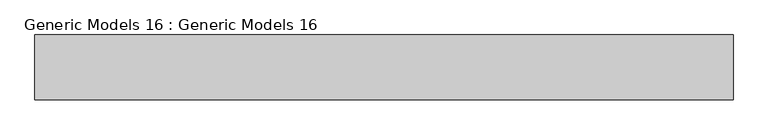
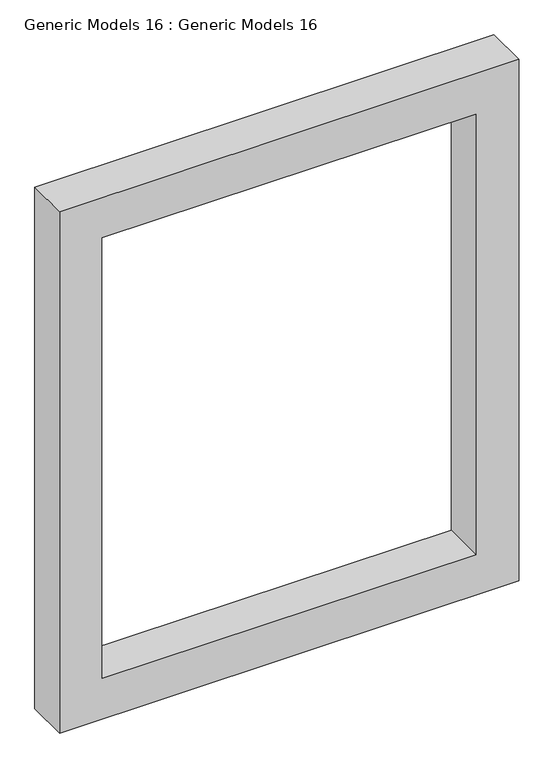
"""IFC4 building model written with IfcOpenShell, lengths in millimetres: proxy geometry, Generic Models 16 : Generic Models 16."""

from ifc_helpers import new_model, si_unit, frame, origin, place, context, project, spatial, polyline, outline, extrude, source, transform, mapped, element, save


def generic_models_16_generic_models_16_40d4eb7f(model_context):
    return source(origin(), model_context, "Body", "SweptSolid", [
        extrude(outline(polyline([(2952.75, -3553.3586008), (987.4676291, -3553.3586008), (987.4676291, -1915.0586008), (2952.75, -1915.0586008), (2952.75, -3553.3586008)]), holes=[polyline([(2800.35, -3400.9586008), (2800.35, -2067.4586008), (1139.8676291, -2067.4586008), (1139.8676291, -3400.9586008), (2800.35, -3400.9586008)])]), frame((0.0, 4970.6155883, 0.0), z_axis=(0.0, 1.0, 0.0), x_axis=(0.0, 0.0, 1.0)), (0.0, 0.0, 1.0), 152.4),
    ])


if __name__ == "__main__":
    model = new_model("IFC4")
    model_context = context("Model", 3, world=origin())
    ifc_project = project(units=[si_unit("LENGTHUNIT", "METRE", prefix="MILLI")], contexts=[model_context])
    site = spatial("IfcSite", under=ifc_project)
    building = spatial("IfcBuilding", under=site)
    placement = place(None, origin())
    generic_models_16_generic_models_16_shape = generic_models_16_generic_models_16_40d4eb7f(model_context)
    element("IfcBuildingElementProxy", 1, Name="Generic Models 16 : Generic Models 16", ObjectType="Generic Models 16 : Generic Models 16", at=placement, inside=building, context=model_context, shape_type="MappedRepresentation", body=[
        mapped(generic_models_16_generic_models_16_shape, transform((0.0, 0.0, 0.0), x_axis=(1.0, 0.0, 0.0), y_axis=(0.0, 1.0, 0.0), z_axis=(0.0, 0.0, 1.0))),
    ])
    save(model, "model.ifc")

# Revit data of these elements
# Element 1 (IfcBuildingElementProxy, "Generic Models 16 : Generic Models 16")
#   Materials on its faces: "feature frame"
# Materials
#   "feature frame": class "Generic", colour RGB 120 120 120, transparency 0, Cost = 0
